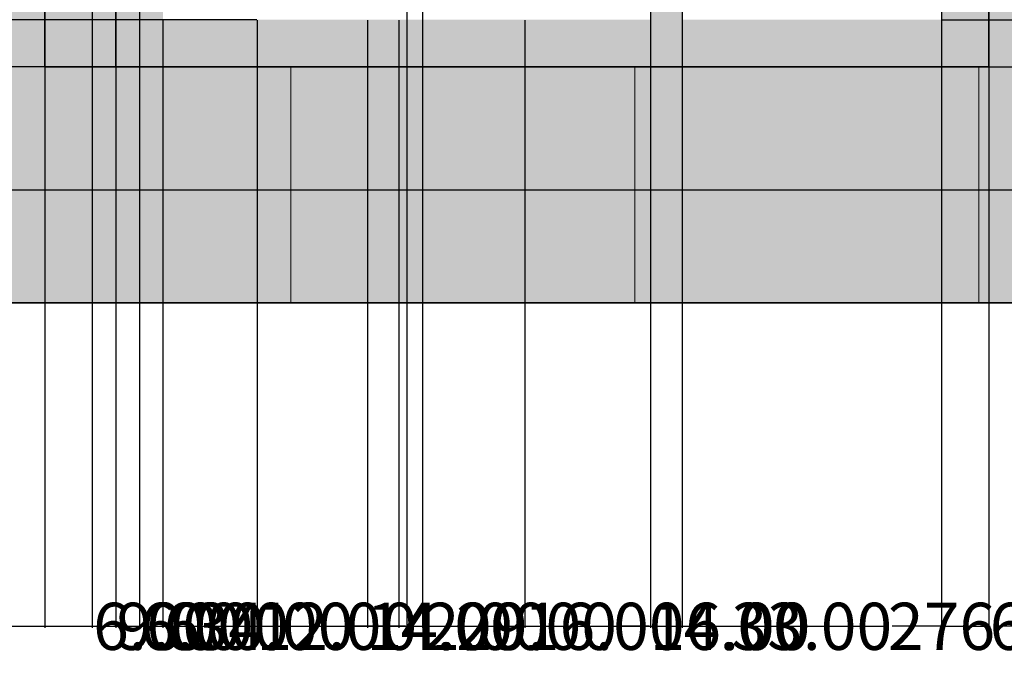
# Model space of a CAD drawing. Units: inches. Extents: x 148 to 1080, y 89 to 707.
# Tile 2 of 12: x 272 to 397, y 89 to 170. Entities that reach past the tile are written whole.
import ezdxf

# ---------------------------------------------------------------- set-up
doc = ezdxf.new("R2010")
doc.units = ezdxf.units.IN
doc.header["$MEASUREMENT"] = 0
for name, color, linetype, lineweight in [('A-ANNO-DIMS', 2, 'Continuous', 18), ('A-ELEV', 7, 'Continuous', 35), ('A-ELEV-PATT', 8, 'Continuous', 13)]:
    doc.layers.add(name, color=color, linetype=linetype, lineweight=lineweight)
doc.styles.get("Standard").update_dxf_attribs({"font": 'arial.ttf'})
doc.dimstyles.get("Standard").update_dxf_attribs({"dimtxt": 6, "dimasz": 0.18, "dimexe": 0.18, "dimexo": 0.0625, "dimgap": 0.09, "dimtad": 0, "dimtih": 1, "dimtoh": 1, "dimdec": 0, "dimzin": 0, "dimdsep": 46, "dimlunit": 3, "dimtxsty": 'Standard', "dimcen": 0.09, "dimadec": 0, "dimazin": 0, "dimtfac": 1, "dimtdec": 0, "dimtofl": 0, "dimtmove": 0, "dimatfit": 3, "dimfxl": 1, "dimtolj": 1, "dimtzin": 0, "dimarcsym": 0})

# ---------------------------------------------------------------- blocks, each defined once
blk = doc.blocks.new('*D2')
at = {"layer": 'A-ANNO-DIMS', "color": 0, "lineweight": -2, "transparency": 16777216}
for p, q in [((251.02, 133.88), (251.02, 92.62)), ((527.02, 133.88), (527.02, 92.62)), ((251.2, 92.8), (382.25, 92.8)), ((526.84, 92.8), (395.79, 92.8))]:
    blk.add_line(p, q, dxfattribs=at)
at = {"layer": 'A-ANNO-DIMS', "color": 0, "transparency": 16777216}
for points in [[(251.2, 92.83), (251.2, 92.77), (251.02, 92.8)], [(526.84, 92.83), (526.84, 92.77), (527.02, 92.8)]]:
    blk.add_solid(points, dxfattribs=at)
at = {"layer": 'Defpoints', "color": 0, "transparency": 16777216}
for p in [(251.02, 133.95), (527.02, 133.95), (527.02, 92.8)]:
    blk.add_point(p, dxfattribs=at)
at = {"layer": 'A-ANNO-DIMS', "color": 0, "transparency": 16777216, "insert": (389.02, 92.8), "char_height": 6, "attachment_point": 5}
blk.add_mtext('\\A1;276', dxfattribs=at)
blk = doc.blocks.new('*D28')
at = {"layer": 'A-ANNO-DIMS', "color": 0, "lineweight": -2, "transparency": 16777216}
for p, q in [((274.96, 331.95), (160.42, 331.95)), ((160.6, 331.77), (160.6, 251.1)), ((160.6, 164.13), (160.6, 244.79)), ((274.96, 163.95), (160.42, 163.95))]:
    blk.add_line(p, q, dxfattribs=at)
at = {"layer": 'A-ANNO-DIMS', "color": 0, "transparency": 16777216}
for points in [[(160.57, 331.77), (160.63, 331.77), (160.6, 331.95)], [(160.57, 164.13), (160.63, 164.13), (160.6, 163.95)]]:
    blk.add_solid(points, dxfattribs=at)
at = {"layer": 'Defpoints', "color": 0, "transparency": 16777216}
for p in [(160.6, 331.95), (275.02, 331.95), (275.02, 163.95)]:
    blk.add_point(p, dxfattribs=at)
at = {"layer": 'A-ANNO-DIMS', "color": 0, "transparency": 16777216, "insert": (160.6, 247.95), "char_height": 6, "attachment_point": 5}
blk.add_mtext('\\A1;168', dxfattribs=at)
blk = doc.blocks.new('*D29')
at = {"layer": 'A-ANNO-DIMS', "color": 0, "lineweight": -2, "transparency": 16777216}
for p, q in [((274.96, 163.95), (160.42, 163.95)), ((160.6, 163.77), (160.6, 152.1)), ((160.6, 134.13), (160.6, 145.79)), ((250.96, 133.95), (160.42, 133.95))]:
    blk.add_line(p, q, dxfattribs=at)
at = {"layer": 'A-ANNO-DIMS', "color": 0, "transparency": 16777216}
for points in [[(160.57, 163.77), (160.63, 163.77), (160.6, 163.95)], [(160.57, 134.13), (160.63, 134.13), (160.6, 133.95)]]:
    blk.add_solid(points, dxfattribs=at)
at = {"layer": 'Defpoints', "color": 0, "transparency": 16777216}
for p in [(275.02, 163.95), (160.6, 133.95), (251.02, 133.95)]:
    blk.add_point(p, dxfattribs=at)
at = {"layer": 'A-ANNO-DIMS', "color": 0, "transparency": 16777216, "insert": (160.6, 148.95), "char_height": 6, "attachment_point": 5}
blk.add_mtext('\\A1;30', dxfattribs=at)
blk = doc.blocks.new('*D32')
at = {"layer": 'A-ANNO-DIMS', "color": 0, "lineweight": -2, "transparency": 16777216}
for p, q in [((587, 271.77), (160.42, 271.77)), ((160.6, 271.59), (160.6, 213.18)), ((160.6, 148.46), (160.6, 206.87)), ((587, 148.28), (160.42, 148.28))]:
    blk.add_line(p, q, dxfattribs=at)
at = {"layer": 'A-ANNO-DIMS', "color": 0, "transparency": 16777216}
for points in [[(160.57, 271.59), (160.63, 271.59), (160.6, 271.77)], [(160.57, 148.46), (160.63, 148.46), (160.6, 148.28)]]:
    blk.add_solid(points, dxfattribs=at)
at = {"layer": 'Defpoints', "color": 0, "transparency": 16777216}
for p in [(160.6, 271.77), (587.06, 271.77), (587.06, 148.28)]:
    blk.add_point(p, dxfattribs=at)
at = {"layer": 'A-ANNO-DIMS', "color": 0, "transparency": 16777216, "insert": (160.6, 210.03), "char_height": 6, "attachment_point": 5}
blk.add_mtext('\\A1;123.5', dxfattribs=at)
blk = doc.blocks.new('*D34')
at = {"layer": 'A-ANNO-DIMS', "color": 0, "lineweight": -2, "transparency": 16777216}
for p, q in [((574.96, 283.95), (160.42, 283.95)), ((160.6, 283.77), (160.6, 212.1)), ((160.6, 134.13), (160.6, 205.79)), ((574.96, 133.95), (160.42, 133.95))]:
    blk.add_line(p, q, dxfattribs=at)
at = {"layer": 'A-ANNO-DIMS', "color": 0, "transparency": 16777216}
for points in [[(160.57, 283.77), (160.63, 283.77), (160.6, 283.95)], [(160.57, 134.13), (160.63, 134.13), (160.6, 133.95)]]:
    blk.add_solid(points, dxfattribs=at)
at = {"layer": 'Defpoints', "color": 0, "transparency": 16777216}
for p in [(575.02, 283.95), (160.6, 133.95), (575.02, 133.95)]:
    blk.add_point(p, dxfattribs=at)
at = {"layer": 'A-ANNO-DIMS', "color": 0, "transparency": 16777216, "insert": (160.6, 208.95), "char_height": 6, "attachment_point": 5}
blk.add_mtext('\\A1;150', dxfattribs=at)
blk = doc.blocks.new('*D38')
at = {"layer": 'A-ANNO-DIMS', "color": 0, "lineweight": -2, "transparency": 16777216}
for p, q in [((934.89, 271.95), (160.42, 271.95)), ((160.6, 271.77), (160.6, 206.1)), ((160.6, 134.13), (160.6, 199.79)), ((934.89, 133.95), (160.42, 133.95))]:
    blk.add_line(p, q, dxfattribs=at)
at = {"layer": 'A-ANNO-DIMS', "color": 0, "transparency": 16777216}
for points in [[(160.57, 271.77), (160.63, 271.77), (160.6, 271.95)], [(160.57, 134.13), (160.63, 134.13), (160.6, 133.95)]]:
    blk.add_solid(points, dxfattribs=at)
at = {"layer": 'Defpoints', "color": 0, "transparency": 16777216}
for p in [(934.95, 271.95), (160.6, 133.95), (934.95, 133.95)]:
    blk.add_point(p, dxfattribs=at)
at = {"layer": 'A-ANNO-DIMS', "color": 0, "transparency": 16777216, "insert": (160.6, 202.95), "char_height": 6, "attachment_point": 5}
blk.add_mtext('\\A1;138', dxfattribs=at)
blk = doc.blocks.new('*D43')
at = {"layer": 'A-ANNO-DIMS', "color": 0, "lineweight": -2, "transparency": 16777216}
for p, q in [((765.88, 241.1), (160.42, 241.1)), ((160.6, 240.92), (160.6, 190.68)), ((160.6, 134.13), (160.6, 184.37)), ((776.65, 133.95), (160.42, 133.95))]:
    blk.add_line(p, q, dxfattribs=at)
at = {"layer": 'A-ANNO-DIMS', "color": 0, "transparency": 16777216}
for points in [[(160.57, 240.92), (160.63, 240.92), (160.6, 241.1)], [(160.57, 134.13), (160.63, 134.13), (160.6, 133.95)]]:
    blk.add_solid(points, dxfattribs=at)
at = {"layer": 'Defpoints', "color": 0, "transparency": 16777216}
for p in [(765.95, 241.1), (160.6, 133.95), (776.71, 133.95)]:
    blk.add_point(p, dxfattribs=at)
at = {"layer": 'A-ANNO-DIMS', "color": 0, "transparency": 16777216, "insert": (160.6, 187.52), "char_height": 6, "attachment_point": 5}
blk.add_mtext('\\A1;107.15', dxfattribs=at)
blk = doc.blocks.new('*D61')
at = {"layer": 'A-ANNO-DIMS', "color": 0, "lineweight": -2, "transparency": 16777216}
for p, q in [((275.02, 163.88), (275.02, 92.62)), ((284.02, 163.88), (284.02, 92.62)), ((275.2, 92.8), (283.84, 92.8)), ((284.02, 92.8), (284.2, 92.8))]:
    blk.add_line(p, q, dxfattribs=at)
at = {"layer": 'A-ANNO-DIMS', "color": 0, "transparency": 16777216}
for points in [[(275.2, 92.83), (275.2, 92.77), (275.02, 92.8)], [(283.84, 92.83), (283.84, 92.77), (284.02, 92.8)]]:
    blk.add_solid(points, dxfattribs=at)
at = {"layer": 'Defpoints', "color": 0, "transparency": 16777216}
for p in [(275.02, 163.95), (284.02, 163.95), (284.02, 92.8)]:
    blk.add_point(p, dxfattribs=at)
at = {"layer": 'A-ANNO-DIMS', "color": 0, "transparency": 16777216, "insert": (292.07, 92.8), "char_height": 6, "attachment_point": 5}
blk.add_mtext('\\A1;9.00', dxfattribs=at)
blk = doc.blocks.new('*D62')
at = {"layer": 'A-ANNO-DIMS', "color": 0, "lineweight": -2, "transparency": 16777216}
for p, q in [((290.02, 169.88), (290.02, 92.62)), ((284.02, 163.88), (284.02, 92.62)), ((284.2, 92.8), (289.84, 92.8)), ((290.02, 92.8), (290.2, 92.8))]:
    blk.add_line(p, q, dxfattribs=at)
at = {"layer": 'A-ANNO-DIMS', "color": 0, "transparency": 16777216}
for points in [[(284.2, 92.83), (284.2, 92.77), (284.02, 92.8)], [(289.84, 92.83), (289.84, 92.77), (290.02, 92.8)]]:
    blk.add_solid(points, dxfattribs=at)
at = {"layer": 'Defpoints', "color": 0, "transparency": 16777216}
for p in [(290.02, 169.95), (284.02, 163.95), (290.02, 92.8)]:
    blk.add_point(p, dxfattribs=at)
at = {"layer": 'A-ANNO-DIMS', "color": 0, "transparency": 16777216, "insert": (298.09, 92.8), "char_height": 6, "attachment_point": 5}
blk.add_mtext('\\A1;6.00', dxfattribs=at)
blk = doc.blocks.new('*D63')
at = {"layer": 'A-ANNO-DIMS', "color": 0, "lineweight": -2, "transparency": 16777216}
for p, q in [((290.02, 169.88), (290.02, 92.62)), ((302.02, 169.88), (302.02, 92.62)), ((290.2, 92.8), (301.84, 92.8)), ((302.02, 92.8), (302.2, 92.8))]:
    blk.add_line(p, q, dxfattribs=at)
at = {"layer": 'A-ANNO-DIMS', "color": 0, "transparency": 16777216}
for points in [[(290.2, 92.83), (290.2, 92.77), (290.02, 92.8)], [(301.84, 92.83), (301.84, 92.77), (302.02, 92.8)]]:
    blk.add_solid(points, dxfattribs=at)
at = {"layer": 'Defpoints', "color": 0, "transparency": 16777216}
for p in [(290.02, 169.95), (302.02, 169.95), (302.02, 92.8)]:
    blk.add_point(p, dxfattribs=at)
at = {"layer": 'A-ANNO-DIMS', "color": 0, "transparency": 16777216, "insert": (312.12, 92.8), "char_height": 6, "attachment_point": 5}
blk.add_mtext('\\A1;12.00', dxfattribs=at)
blk = doc.blocks.new('*D64')
at = {"layer": 'A-ANNO-DIMS', "color": 0, "lineweight": -2, "transparency": 16777216}
for p, q in [((302.02, 169.88), (302.02, 92.62)), ((316.02, 169.88), (316.02, 92.62)), ((302.2, 92.8), (315.84, 92.8)), ((316.02, 92.8), (316.2, 92.8))]:
    blk.add_line(p, q, dxfattribs=at)
at = {"layer": 'A-ANNO-DIMS', "color": 0, "transparency": 16777216}
for points in [[(302.2, 92.83), (302.2, 92.77), (302.02, 92.8)], [(315.84, 92.83), (315.84, 92.77), (316.02, 92.8)]]:
    blk.add_solid(points, dxfattribs=at)
at = {"layer": 'Defpoints', "color": 0, "transparency": 16777216}
for p in [(302.02, 169.95), (316.02, 169.95), (316.02, 92.8)]:
    blk.add_point(p, dxfattribs=at)
at = {"layer": 'A-ANNO-DIMS', "color": 0, "transparency": 16777216, "insert": (326.12, 92.8), "char_height": 6, "attachment_point": 5}
blk.add_mtext('\\A1;14.00', dxfattribs=at)
blk = doc.blocks.new('*D65')
at = {"layer": 'A-ANNO-DIMS', "color": 0, "lineweight": -2, "transparency": 16777216}
for p, q in [((316.02, 169.88), (316.02, 92.62)), ((320.02, 169.88), (320.02, 92.62)), ((316.2, 92.8), (319.84, 92.8)), ((320.02, 92.8), (320.2, 92.8))]:
    blk.add_line(p, q, dxfattribs=at)
at = {"layer": 'A-ANNO-DIMS', "color": 0, "transparency": 16777216}
for points in [[(316.2, 92.83), (316.2, 92.77), (316.02, 92.8)], [(319.84, 92.83), (319.84, 92.77), (320.02, 92.8)]]:
    blk.add_solid(points, dxfattribs=at)
at = {"layer": 'Defpoints', "color": 0, "transparency": 16777216}
for p in [(316.02, 169.95), (320.02, 169.95), (320.02, 92.8)]:
    blk.add_point(p, dxfattribs=at)
at = {"layer": 'A-ANNO-DIMS', "color": 0, "transparency": 16777216, "insert": (328.19, 92.8), "char_height": 6, "attachment_point": 5}
blk.add_mtext('\\A1;4.00', dxfattribs=at)
blk = doc.blocks.new('*D66')
at = {"layer": 'A-ANNO-DIMS', "color": 0, "lineweight": -2, "transparency": 16777216}
for p, q in [((320.02, 169.88), (320.02, 92.62)), ((336.02, 169.88), (336.02, 92.62)), ((320.2, 92.8), (335.84, 92.8)), ((336.02, 92.8), (336.2, 92.8))]:
    blk.add_line(p, q, dxfattribs=at)
at = {"layer": 'A-ANNO-DIMS', "color": 0, "transparency": 16777216}
for points in [[(320.2, 92.83), (320.2, 92.77), (320.02, 92.8)], [(335.84, 92.83), (335.84, 92.77), (336.02, 92.8)]]:
    blk.add_solid(points, dxfattribs=at)
at = {"layer": 'Defpoints', "color": 0, "transparency": 16777216}
for p in [(320.02, 169.95), (336.02, 169.95), (336.02, 92.8)]:
    blk.add_point(p, dxfattribs=at)
at = {"layer": 'A-ANNO-DIMS', "color": 0, "transparency": 16777216, "insert": (346.12, 92.8), "char_height": 6, "attachment_point": 5}
blk.add_mtext('\\A1;16.00', dxfattribs=at)
blk = doc.blocks.new('*D67')
at = {"layer": 'A-ANNO-DIMS', "color": 0, "lineweight": -2, "transparency": 16777216}
for p, q in [((336.02, 169.88), (336.02, 92.62)), ((352.02, 169.88), (352.02, 92.62)), ((336.2, 92.8), (351.84, 92.8)), ((352.02, 92.8), (352.2, 92.8))]:
    blk.add_line(p, q, dxfattribs=at)
at = {"layer": 'A-ANNO-DIMS', "color": 0, "transparency": 16777216}
for points in [[(336.2, 92.83), (336.2, 92.77), (336.02, 92.8)], [(351.84, 92.83), (351.84, 92.77), (352.02, 92.8)]]:
    blk.add_solid(points, dxfattribs=at)
at = {"layer": 'Defpoints', "color": 0, "transparency": 16777216}
for p in [(336.02, 169.95), (352.02, 169.95), (352.02, 92.8)]:
    blk.add_point(p, dxfattribs=at)
at = {"layer": 'A-ANNO-DIMS', "color": 0, "transparency": 16777216, "insert": (362.12, 92.8), "char_height": 6, "attachment_point": 5}
blk.add_mtext('\\A1;16.00', dxfattribs=at)
blk = doc.blocks.new('*D68')
at = {"layer": 'A-ANNO-DIMS', "color": 0, "lineweight": -2, "transparency": 16777216}
for p, q in [((352.02, 169.88), (352.02, 92.62)), ((356.02, 169.88), (356.02, 92.62)), ((352.2, 92.8), (355.84, 92.8)), ((356.02, 92.8), (356.2, 92.8))]:
    blk.add_line(p, q, dxfattribs=at)
at = {"layer": 'A-ANNO-DIMS', "color": 0, "transparency": 16777216}
for points in [[(352.2, 92.83), (352.2, 92.77), (352.02, 92.8)], [(355.84, 92.83), (355.84, 92.77), (356.02, 92.8)]]:
    blk.add_solid(points, dxfattribs=at)
at = {"layer": 'Defpoints', "color": 0, "transparency": 16777216}
for p in [(352.02, 169.95), (356.02, 169.95), (356.02, 92.8)]:
    blk.add_point(p, dxfattribs=at)
at = {"layer": 'A-ANNO-DIMS', "color": 0, "transparency": 16777216, "insert": (364.19, 92.8), "char_height": 6, "attachment_point": 5}
blk.add_mtext('\\A1;4.00', dxfattribs=at)
blk = doc.blocks.new('*D69')
at = {"layer": 'A-ANNO-DIMS', "color": 0, "lineweight": -2, "transparency": 16777216}
for p, q in [((356.02, 169.88), (356.02, 92.62)), ((389.02, 169.88), (389.02, 92.62)), ((356.2, 92.8), (362.32, 92.8)), ((388.84, 92.8), (382.72, 92.8))]:
    blk.add_line(p, q, dxfattribs=at)
at = {"layer": 'A-ANNO-DIMS', "color": 0, "transparency": 16777216}
for points in [[(356.2, 92.83), (356.2, 92.77), (356.02, 92.8)], [(388.84, 92.83), (388.84, 92.77), (389.02, 92.8)]]:
    blk.add_solid(points, dxfattribs=at)
at = {"layer": 'Defpoints', "color": 0, "transparency": 16777216}
for p in [(356.02, 169.95), (389.02, 169.95), (389.02, 92.8)]:
    blk.add_point(p, dxfattribs=at)
at = {"layer": 'A-ANNO-DIMS', "color": 0, "transparency": 16777216, "insert": (372.52, 92.8), "char_height": 6, "attachment_point": 5}
blk.add_mtext('\\A1;33.00', dxfattribs=at)
blk = doc.blocks.new('*D70')
at = {"layer": 'A-ANNO-DIMS', "color": 0, "lineweight": -2, "transparency": 16777216}
for p, q in [((389.02, 169.88), (389.02, 92.62)), ((395.02, 163.88), (395.02, 92.62)), ((389.2, 92.8), (394.84, 92.8)), ((395.02, 92.8), (395.2, 92.8))]:
    blk.add_line(p, q, dxfattribs=at)
at = {"layer": 'A-ANNO-DIMS', "color": 0, "transparency": 16777216}
for points in [[(389.2, 92.83), (389.2, 92.77), (389.02, 92.8)], [(394.84, 92.83), (394.84, 92.77), (395.02, 92.8)]]:
    blk.add_solid(points, dxfattribs=at)
at = {"layer": 'Defpoints', "color": 0, "transparency": 16777216}
for p in [(389.02, 169.95), (395.02, 163.95), (395.02, 92.8)]:
    blk.add_point(p, dxfattribs=at)
at = {"layer": 'A-ANNO-DIMS', "color": 0, "transparency": 16777216, "insert": (403.09, 92.8), "char_height": 6, "attachment_point": 5}
blk.add_mtext('\\A1;6.00', dxfattribs=at)
blk = doc.blocks.new('*D71')
at = {"layer": 'A-ANNO-DIMS', "color": 0, "lineweight": -2, "transparency": 16777216}
for p, q in [((389.08, 169.95), (1064.5, 169.95)), ((1064.32, 169.95), (1064.32, 170.13)), ((1064.32, 170.13), (1064.5, 170.13)), ((1064.32, 164.13), (1064.32, 169.77)), ((395.08, 163.95), (1064.5, 163.95))]:
    blk.add_line(p, q, dxfattribs=at)
at = {"layer": 'A-ANNO-DIMS', "color": 0, "transparency": 16777216}
for points in [[(1064.29, 169.77), (1064.35, 169.77), (1064.32, 169.95)], [(1064.29, 164.13), (1064.35, 164.13), (1064.32, 163.95)]]:
    blk.add_solid(points, dxfattribs=at)
at = {"layer": 'Defpoints', "color": 0, "transparency": 16777216}
for p in [(389.02, 169.95), (1064.32, 169.95), (395.02, 163.95)]:
    blk.add_point(p, dxfattribs=at)
at = {"layer": 'A-ANNO-DIMS', "color": 0, "transparency": 16777216, "insert": (1072.39, 170.13), "char_height": 6, "attachment_point": 5}
blk.add_mtext('\\A1;6.00', dxfattribs=at)
blk = doc.blocks.new('*D72')
at = {"layer": 'A-ANNO-DIMS', "color": 0, "lineweight": -2, "transparency": 16777216}
for p, q in [((389.08, 192.87), (1064.5, 192.87)), ((1064.32, 192.69), (1064.32, 184.56)), ((1064.32, 170.13), (1064.32, 178.26)), ((389.08, 169.95), (1064.5, 169.95))]:
    blk.add_line(p, q, dxfattribs=at)
at = {"layer": 'A-ANNO-DIMS', "color": 0, "transparency": 16777216}
for points in [[(1064.29, 192.69), (1064.35, 192.69), (1064.32, 192.87)], [(1064.29, 170.13), (1064.35, 170.13), (1064.32, 169.95)]]:
    blk.add_solid(points, dxfattribs=at)
at = {"layer": 'Defpoints', "color": 0, "transparency": 16777216}
for p in [(389.02, 192.87), (1064.32, 192.87), (389.02, 169.95)]:
    blk.add_point(p, dxfattribs=at)
at = {"layer": 'A-ANNO-DIMS', "color": 0, "transparency": 16777216, "insert": (1064.32, 181.41), "char_height": 6, "attachment_point": 5}
blk.add_mtext('\\A1;22.92', dxfattribs=at)
blk = doc.blocks.new('*D80')
at = {"layer": 'A-ANNO-DIMS', "color": 0, "lineweight": -2, "transparency": 16777216}
for p, q in [((289.96, 222.32), (160.42, 222.32)), ((160.6, 222.14), (160.6, 199.29)), ((160.6, 170.13), (160.6, 192.98)), ((289.96, 169.95), (160.42, 169.95))]:
    blk.add_line(p, q, dxfattribs=at)
at = {"layer": 'A-ANNO-DIMS', "color": 0, "transparency": 16777216}
for points in [[(160.57, 222.14), (160.63, 222.14), (160.6, 222.32)], [(160.57, 170.13), (160.63, 170.13), (160.6, 169.95)]]:
    blk.add_solid(points, dxfattribs=at)
at = {"layer": 'Defpoints', "color": 0, "transparency": 16777216}
for p in [(160.6, 222.32), (290.02, 222.32), (290.02, 169.95)]:
    blk.add_point(p, dxfattribs=at)
at = {"layer": 'A-ANNO-DIMS', "color": 0, "transparency": 16777216, "insert": (160.6, 196.13), "char_height": 6, "attachment_point": 5}
blk.add_mtext('\\A1;52.37', dxfattribs=at)
blk = doc.blocks.new('*D81')
at = {"layer": 'A-ANNO-DIMS', "color": 0, "lineweight": -2, "transparency": 16777216}
for p, q in [((301.96, 206.89), (160.42, 206.89)), ((160.6, 206.71), (160.6, 191.57)), ((160.6, 170.13), (160.6, 185.26)), ((301.96, 169.95), (160.42, 169.95))]:
    blk.add_line(p, q, dxfattribs=at)
at = {"layer": 'A-ANNO-DIMS', "color": 0, "transparency": 16777216}
for points in [[(160.57, 206.71), (160.63, 206.71), (160.6, 206.89)], [(160.57, 170.13), (160.63, 170.13), (160.6, 169.95)]]:
    blk.add_solid(points, dxfattribs=at)
at = {"layer": 'Defpoints', "color": 0, "transparency": 16777216}
for p in [(160.6, 206.89), (302.02, 206.89), (302.02, 169.95)]:
    blk.add_point(p, dxfattribs=at)
at = {"layer": 'A-ANNO-DIMS', "color": 0, "transparency": 16777216, "insert": (160.6, 188.42), "char_height": 6, "attachment_point": 5}
blk.add_mtext('\\A1;36.944', dxfattribs=at)
blk = doc.blocks.new('*D82')
at = {"layer": 'A-ANNO-DIMS', "color": 0, "lineweight": -2, "transparency": 16777216}
for p, q in [((275.02, 400.88), (275.02, 92.62)), ((281.02, 400.88), (281.02, 92.62)), ((275.2, 92.8), (280.84, 92.8)), ((281.02, 92.8), (281.2, 92.8))]:
    blk.add_line(p, q, dxfattribs=at)
at = {"layer": 'A-ANNO-DIMS', "color": 0, "transparency": 16777216}
for points in [[(275.2, 92.83), (275.2, 92.77), (275.02, 92.8)], [(280.84, 92.83), (280.84, 92.77), (281.02, 92.8)]]:
    blk.add_solid(points, dxfattribs=at)
at = {"layer": 'Defpoints', "color": 0, "transparency": 16777216}
for p in [(275.02, 400.95), (281.02, 400.95), (281.02, 92.8)]:
    blk.add_point(p, dxfattribs=at)
at = {"layer": 'A-ANNO-DIMS', "color": 0, "transparency": 16777216, "insert": (289.09, 92.8), "char_height": 6, "attachment_point": 5}
blk.add_mtext('\\A1;6.00', dxfattribs=at)
blk = doc.blocks.new('*D83')
at = {"layer": 'A-ANNO-DIMS', "color": 0, "lineweight": -2, "transparency": 16777216}
for p, q in [((281.02, 400.88), (281.02, 92.62)), ((287.02, 400.88), (287.02, 92.62)), ((281.2, 92.8), (286.84, 92.8)), ((287.02, 92.8), (287.2, 92.8))]:
    blk.add_line(p, q, dxfattribs=at)
at = {"layer": 'A-ANNO-DIMS', "color": 0, "transparency": 16777216}
for points in [[(281.2, 92.83), (281.2, 92.77), (281.02, 92.8)], [(286.84, 92.83), (286.84, 92.77), (287.02, 92.8)]]:
    blk.add_solid(points, dxfattribs=at)
at = {"layer": 'Defpoints', "color": 0, "transparency": 16777216}
for p in [(281.02, 400.95), (287.02, 400.95), (287.02, 92.8)]:
    blk.add_point(p, dxfattribs=at)
at = {"layer": 'A-ANNO-DIMS', "color": 0, "transparency": 16777216, "insert": (295.09, 92.8), "char_height": 6, "attachment_point": 5}
blk.add_mtext('\\A1;6.00', dxfattribs=at)
blk = doc.blocks.new('*D84')
at = {"layer": 'A-ANNO-DIMS', "color": 0, "lineweight": -2, "transparency": 16777216}
for p, q in [((321.02, 529.88), (321.02, 92.62)), ((287.02, 400.88), (287.02, 92.62)), ((287.2, 92.8), (293.82, 92.8)), ((320.84, 92.8), (314.22, 92.8))]:
    blk.add_line(p, q, dxfattribs=at)
at = {"layer": 'A-ANNO-DIMS', "color": 0, "transparency": 16777216}
for points in [[(287.2, 92.83), (287.2, 92.77), (287.02, 92.8)], [(320.84, 92.83), (320.84, 92.77), (321.02, 92.8)]]:
    blk.add_solid(points, dxfattribs=at)
at = {"layer": 'Defpoints', "color": 0, "transparency": 16777216}
for p in [(321.02, 529.95), (287.02, 400.95), (321.02, 92.8)]:
    blk.add_point(p, dxfattribs=at)
at = {"layer": 'A-ANNO-DIMS', "color": 0, "transparency": 16777216, "insert": (304.02, 92.8), "char_height": 6, "attachment_point": 5}
blk.add_mtext('\\A1;34.00', dxfattribs=at)
blk = doc.blocks.new('*D85')
at = {"layer": 'A-ANNO-DIMS', "color": 0, "lineweight": -2, "transparency": 16777216}
for p, q in [((321.02, 529.88), (321.02, 92.62)), ((323.02, 400.88), (323.02, 92.62)), ((321.2, 92.8), (322.84, 92.8)), ((323.02, 92.8), (323.2, 92.8))]:
    blk.add_line(p, q, dxfattribs=at)
at = {"layer": 'A-ANNO-DIMS', "color": 0, "transparency": 16777216}
for points in [[(321.2, 92.83), (321.2, 92.77), (321.02, 92.8)], [(322.84, 92.83), (322.84, 92.77), (323.02, 92.8)]]:
    blk.add_solid(points, dxfattribs=at)
at = {"layer": 'Defpoints', "color": 0, "transparency": 16777216}
for p in [(321.02, 529.95), (323.02, 400.95), (323.02, 92.8)]:
    blk.add_point(p, dxfattribs=at)
at = {"layer": 'A-ANNO-DIMS', "color": 0, "transparency": 16777216, "insert": (331.12, 92.8), "char_height": 6, "attachment_point": 5}
blk.add_mtext('\\A1;2.00', dxfattribs=at)
blk = doc.blocks.new('*D86')
at = {"layer": 'A-ANNO-DIMS', "color": 0, "lineweight": -2, "transparency": 16777216}
for p, q in [((323.02, 400.88), (323.02, 92.62)), ((352.02, 400.88), (352.02, 92.62)), ((323.2, 92.8), (327.27, 92.8)), ((351.84, 92.8), (347.77, 92.8))]:
    blk.add_line(p, q, dxfattribs=at)
at = {"layer": 'A-ANNO-DIMS', "color": 0, "transparency": 16777216}
for points in [[(323.2, 92.83), (323.2, 92.77), (323.02, 92.8)], [(351.84, 92.83), (351.84, 92.77), (352.02, 92.8)]]:
    blk.add_solid(points, dxfattribs=at)
at = {"layer": 'Defpoints', "color": 0, "transparency": 16777216}
for p in [(323.02, 400.95), (352.02, 400.95), (352.02, 92.8)]:
    blk.add_point(p, dxfattribs=at)
at = {"layer": 'A-ANNO-DIMS', "color": 0, "transparency": 16777216, "insert": (337.52, 92.8), "char_height": 6, "attachment_point": 5}
blk.add_mtext('\\A1;29.00', dxfattribs=at)
blk = doc.blocks.new('*D87')
at = {"layer": 'A-ANNO-DIMS', "color": 0, "lineweight": -2, "transparency": 16777216}
for p, q in [((352.02, 400.88), (352.02, 92.62)), ((356.02, 400.88), (356.02, 92.62)), ((352.2, 92.8), (355.84, 92.8)), ((356.02, 92.8), (356.2, 92.8))]:
    blk.add_line(p, q, dxfattribs=at)
at = {"layer": 'A-ANNO-DIMS', "color": 0, "transparency": 16777216}
for points in [[(352.2, 92.83), (352.2, 92.77), (352.02, 92.8)], [(355.84, 92.83), (355.84, 92.77), (356.02, 92.8)]]:
    blk.add_solid(points, dxfattribs=at)
at = {"layer": 'Defpoints', "color": 0, "transparency": 16777216}
for p in [(352.02, 400.95), (356.02, 400.95), (356.02, 92.8)]:
    blk.add_point(p, dxfattribs=at)
at = {"layer": 'A-ANNO-DIMS', "color": 0, "transparency": 16777216, "insert": (364.19, 92.8), "char_height": 6, "attachment_point": 5}
blk.add_mtext('\\A1;4.00', dxfattribs=at)
blk = doc.blocks.new('*D88')
at = {"layer": 'A-ANNO-DIMS', "color": 0, "lineweight": -2, "transparency": 16777216}
for p, q in [((356.02, 400.88), (356.02, 92.62)), ((389.02, 400.88), (389.02, 92.62)), ((356.2, 92.8), (362.32, 92.8)), ((388.84, 92.8), (382.72, 92.8))]:
    blk.add_line(p, q, dxfattribs=at)
at = {"layer": 'A-ANNO-DIMS', "color": 0, "transparency": 16777216}
for points in [[(356.2, 92.83), (356.2, 92.77), (356.02, 92.8)], [(388.84, 92.83), (388.84, 92.77), (389.02, 92.8)]]:
    blk.add_solid(points, dxfattribs=at)
at = {"layer": 'Defpoints', "color": 0, "transparency": 16777216}
for p in [(356.02, 400.95), (389.02, 400.95), (389.02, 92.8)]:
    blk.add_point(p, dxfattribs=at)
at = {"layer": 'A-ANNO-DIMS', "color": 0, "transparency": 16777216, "insert": (372.52, 92.8), "char_height": 6, "attachment_point": 5}
blk.add_mtext('\\A1;33.00', dxfattribs=at)
blk = doc.blocks.new('*D89')
at = {"layer": 'A-ANNO-DIMS', "color": 0, "lineweight": -2, "transparency": 16777216}
for p, q in [((389.02, 400.88), (389.02, 92.62)), ((395.02, 400.88), (395.02, 92.62)), ((389.2, 92.8), (394.84, 92.8)), ((395.02, 92.8), (395.2, 92.8))]:
    blk.add_line(p, q, dxfattribs=at)
at = {"layer": 'A-ANNO-DIMS', "color": 0, "transparency": 16777216}
for points in [[(389.2, 92.83), (389.2, 92.77), (389.02, 92.8)], [(394.84, 92.83), (394.84, 92.77), (395.02, 92.8)]]:
    blk.add_solid(points, dxfattribs=at)
at = {"layer": 'Defpoints', "color": 0, "transparency": 16777216}
for p in [(389.02, 400.95), (395.02, 400.95), (395.02, 92.8)]:
    blk.add_point(p, dxfattribs=at)
at = {"layer": 'A-ANNO-DIMS', "color": 0, "transparency": 16777216, "insert": (403.09, 92.8), "char_height": 6, "attachment_point": 5}
blk.add_mtext('\\A1;6.00', dxfattribs=at)

msp = doc.modelspace()

# ---------------------------------------------------------------- hatches: boundary and pattern name
at = {"layer": 'A-ELEV-PATT'}
h = msp.add_hatch(color=256, dxfattribs=at)
h.dxf.hatch_style = 1
h.paths.add_polyline_path([(395.0199, 349.9474), (275.0199, 349.9474), (275.0199, 331.9474), (395.0199, 331.9474)])
h.paths.add_polyline_path([(284.0199, 331.9474), (275.0199, 331.9474), (275.0199, 163.9474), (284.0199, 163.9474)])
h.paths.add_polyline_path([(395.0199, 601.9474), (251.0199, 601.9474), (251.0199, 589.9474), (395.0199, 589.9474)])
h = msp.add_hatch(dxfattribs=at)
h.set_pattern_fill('ANSI37', color=256, scale=350, angle=135)
h.paths.add_polyline_path([(527.0199, 349.9474), (395.0199, 349.9474), (395.0199, 163.9474), (275.0199, 163.9474), (275.0199, 349.9474), (251.0199, 349.9474), (251.0199, 133.9474), (527.0199, 133.9474)])
h = msp.add_hatch(color=256, dxfattribs=at)
h.dxf.hatch_style = 1
h.paths.add_polyline_path([(527.0199, 272.3839), (395.0199, 271.2774), (395.0199, 163.9474), (275.0199, 163.9474), (275.0199, 270.2716), (251.0199, 270.0704), (251.0199, 133.9474), (527.0199, 133.9474)])
h.paths.add_polyline_path([(1006.9492, 337.9474), (946.9492, 337.9474), (946.9492, 277.9474), (1006.9492, 277.9474)])
h.paths.add_polyline_path([(1006.9492, 277.9474), (946.9492, 277.9474), (946.9492, 133.9474), (1006.9492, 133.9474)])
h.paths.add_polyline_path([(946.9492, 337.9474), (743.0199, 337.9474), (743.0199, 277.9474), (946.9492, 277.9474)])
h = msp.add_hatch(color=256, dxfattribs=at)
h.dxf.hatch_style = 1
h.paths.add_polyline_path([(290.0199, 331.9474), (284.0199, 331.9474), (284.0199, 163.9474), (395.0199, 163.9474), (395.0199, 331.9474), (290.0199, 331.9474), (290.0199, 325.9474), (352.0199, 325.9474), (352.0199, 304.9474), (356.0199, 304.9474), (356.0199, 325.9474), (389.0199, 325.9474), (389.0199, 169.9474), (290.0199, 169.9474)])
h.paths.add_polyline_path([(356.0199, 300.9474), (352.0199, 300.9474), (352.0199, 169.9474), (356.0199, 169.9474)], flags=17)
h.paths.add_polyline_path([(356.0199, 304.9474), (352.0199, 304.9474), (352.0199, 300.9474), (356.0199, 300.9474)], flags=17)

# ---------------------------------------------------------------- linework, layer by layer
at = {"layer": 'A-ELEV'}
for p, q in [((275.0199, 163.9474), (275.0199, 349.9474)), ((395.0199, 163.9474), (395.0199, 349.9474)), ((284.0199, 163.9474), (284.0199, 331.9474)), ((275.0199, 163.9474), (395.0199, 163.9474)), ((201.7492, 133.9474), (1023.175, 133.9474))]:
    msp.add_line(p, q, dxfattribs=at)

# ---------------------------------------------------------------- dimensions: what is measured, and where the dimension line sits
at = {"layer": 'A-ANNO-DIMS'}
for base, p1, p2, override, picture, middle in [((321.0199, 92.7974), (287.0199, 400.9474), (321.0199, 529.9474), {"dimdec": 2, "dimlfac": 1, "dimrnd": 0, "dimzin": 0, "dimdsep": 46, "dimlunit": 2}, '*D84', (304.0199, 92.7974)), ((323.0199, 92.7974), (321.0199, 529.9474), (323.0199, 400.9474), {"dimdec": 2, "dimlfac": 1, "dimrnd": 0, "dimzin": 0, "dimdsep": 46, "dimlunit": 2}, '*D85', (331.1234, 92.7974)), ((281.0199, 92.7974), (275.0199, 400.9474), (281.0199, 400.9474), {"dimdec": 2, "dimlfac": 1, "dimrnd": 0, "dimzin": 0, "dimdsep": 46, "dimlunit": 2}, '*D82', (289.0886, 92.7974)), ((287.0199, 92.7974), (281.0199, 400.9474), (287.0199, 400.9474), {"dimdec": 2, "dimlfac": 1, "dimrnd": 0, "dimzin": 0, "dimdsep": 46, "dimlunit": 2}, '*D83', (295.0886, 92.7974)), ((352.0199, 92.7974), (323.0199, 400.9474), (352.0199, 400.9474), {"dimdec": 2, "dimlfac": 1, "dimrnd": 0, "dimzin": 0, "dimdsep": 46, "dimlunit": 2}, '*D86', (337.5199, 92.7974)), ((356.0199, 92.7974), (352.0199, 400.9474), (356.0199, 400.9474), {"dimdec": 2, "dimlfac": 1, "dimrnd": 0, "dimzin": 0, "dimdsep": 46, "dimlunit": 2}, '*D87', (364.193, 92.7974)), ((389.0199, 92.7974), (356.0199, 400.9474), (389.0199, 400.9474), {"dimdec": 2, "dimlfac": 1, "dimrnd": 0, "dimzin": 0, "dimdsep": 46, "dimlunit": 2}, '*D88', (372.5199, 92.7974)), ((395.0199, 92.7974), (389.0199, 400.9474), (395.0199, 400.9474), {"dimdec": 2, "dimlfac": 1, "dimrnd": 0, "dimzin": 0, "dimdsep": 46, "dimlunit": 2}, '*D89', (403.0886, 92.7974)), ((290.0199, 92.7974), (284.0199, 163.9474), (290.0199, 169.9474), {"dimdec": 2, "dimlfac": 1, "dimrnd": 0, "dimzin": 0, "dimdsep": 46, "dimlunit": 2}, '*D62', (298.0886, 92.7974)), ((302.0199, 92.7974), (290.0199, 169.9474), (302.0199, 169.9474), {"dimdec": 2, "dimlfac": 1, "dimrnd": 0, "dimzin": 0, "dimdsep": 46, "dimlunit": 2}, '*D63', (312.1207, 92.7974)), ((316.0199, 92.7974), (302.0199, 169.9474), (316.0199, 169.9474), {"dimdec": 2, "dimlfac": 1, "dimrnd": 0, "dimzin": 0, "dimdsep": 46, "dimlunit": 2}, '*D64', (326.1207, 92.7974)), ((320.0199, 92.7974), (316.0199, 169.9474), (320.0199, 169.9474), {"dimdec": 2, "dimlfac": 1, "dimrnd": 0, "dimzin": 0, "dimdsep": 46, "dimlunit": 2}, '*D65', (328.193, 92.7974)), ((336.0199, 92.7974), (320.0199, 169.9474), (336.0199, 169.9474), {"dimdec": 2, "dimlfac": 1, "dimrnd": 0, "dimzin": 0, "dimdsep": 46, "dimlunit": 2}, '*D66', (346.1207, 92.7974)), ((352.0199, 92.7974), (336.0199, 169.9474), (352.0199, 169.9474), {"dimdec": 2, "dimlfac": 1, "dimrnd": 0, "dimzin": 0, "dimdsep": 46, "dimlunit": 2}, '*D67', (362.1207, 92.7974)), ((356.0199, 92.7974), (352.0199, 169.9474), (356.0199, 169.9474), {"dimdec": 2, "dimlfac": 1, "dimrnd": 0, "dimzin": 0, "dimdsep": 46, "dimlunit": 2}, '*D68', (364.193, 92.7974)), ((389.0199, 92.7974), (356.0199, 169.9474), (389.0199, 169.9474), {"dimdec": 2, "dimlfac": 1, "dimrnd": 0, "dimzin": 0, "dimdsep": 46, "dimlunit": 2}, '*D69', (372.5199, 92.7974)), ((395.0199, 92.7974), (389.0199, 169.9474), (395.0199, 163.9474), {"dimdec": 2, "dimlfac": 1, "dimrnd": 0, "dimzin": 0, "dimdsep": 46, "dimlunit": 2}, '*D70', (403.0886, 92.7974)), ((284.0199, 92.7974), (275.0199, 163.9474), (284.0199, 163.9474), {"dimdec": 2, "dimlfac": 1, "dimrnd": 0, "dimzin": 0, "dimdsep": 46, "dimlunit": 2}, '*D61', (292.0723, 92.7974)), ((527.0199, 92.7974), (251.0199, 133.9474), (527.0199, 133.9474), {"dimdec": 0, "dimlfac": 1, "dimrnd": 0, "dimzin": 0, "dimdsep": 46, "dimlunit": 2}, '*D2', (389.0199, 92.7974))]:
    dim = msp.add_linear_dim(base=base, p1=p1, p2=p2, dimstyle='Standard', override=override, dxfattribs=at)
    dim.commit()
    dim.dimension.update_dxf_attribs({"geometry": picture, "text_midpoint": middle})
for base, p1, p2, override, picture, middle in [((160.5992, 331.9474), (275.0199, 163.9474), (275.0199, 331.9474), {"dimdec": 0, "dimlfac": 1, "dimrnd": 0, "dimzin": 0, "dimdsep": 46, "dimlunit": 2}, '*D28', (160.5992, 247.9474)), ((160.5992, 133.9474), (575.0199, 283.9474), (575.0199, 133.9474), {"dimdec": 0, "dimlfac": 1, "dimrnd": 0, "dimzin": 0, "dimdsep": 46, "dimlunit": 2}, '*D34', (160.5992, 208.9474)), ((160.5992, 271.7747), (587.0631, 148.2809), (587.0631, 271.7747), {"dimdec": 1, "dimlfac": 1, "dimrnd": 0, "dimzin": 0, "dimdsep": 46, "dimlunit": 2}, '*D32', (160.5992, 210.0278)), ((160.5992, 133.9474), (934.9492, 271.9474), (934.9492, 133.9474), {"dimdec": 0, "dimlfac": 1, "dimrnd": 0, "dimzin": 0, "dimdsep": 46, "dimlunit": 2}, '*D38', (160.5992, 202.9474)), ((160.5992, 133.9474), (765.9474, 241.0996), (776.713, 133.9474), {"dimdec": 2, "dimlfac": 1, "dimrnd": 0, "dimzin": 0, "dimdsep": 46, "dimlunit": 2}, '*D43', (160.5992, 187.5235)), ((160.5992, 222.3199), (290.0199, 169.9474), (290.0199, 222.3199), {"dimdec": 2, "dimlfac": 1, "dimrnd": 0, "dimzin": 0, "dimdsep": 46, "dimlunit": 2}, '*D80', (160.5992, 196.1336)), ((160.5992, 206.8913), (302.0199, 169.9474), (302.0199, 206.8913), {"dimdec": 3, "dimlfac": 1, "dimrnd": 0, "dimzin": 0, "dimdsep": 46, "dimlunit": 2}, '*D81', (160.5992, 188.4194)), ((1064.325, 192.8696), (389.0199, 169.9474), (389.0199, 192.8696), {"dimdec": 2, "dimlfac": 1, "dimrnd": 0, "dimzin": 0, "dimdsep": 46, "dimlunit": 2}, '*D72', (1064.325, 181.4085)), ((1064.325, 169.9474), (395.0199, 163.9474), (389.0199, 169.9474), {"dimdec": 2, "dimlfac": 1, "dimrnd": 0, "dimzin": 0, "dimdsep": 46, "dimlunit": 2}, '*D71', (1072.3937, 170.1274)), ((160.5992, 133.9474), (275.0199, 163.9474), (251.0199, 133.9474), {"dimdec": 0, "dimlfac": 1, "dimrnd": 0, "dimzin": 0, "dimdsep": 46, "dimlunit": 2}, '*D29', (160.5992, 148.9474))]:
    dim = msp.add_linear_dim(base=base, p1=p1, p2=p2, angle=90, dimstyle='Standard', override=override, dxfattribs=at)
    dim.commit()
    dim.dimension.update_dxf_attribs({"geometry": picture, "text_midpoint": middle})

doc.saveas('drawing.dxf')
